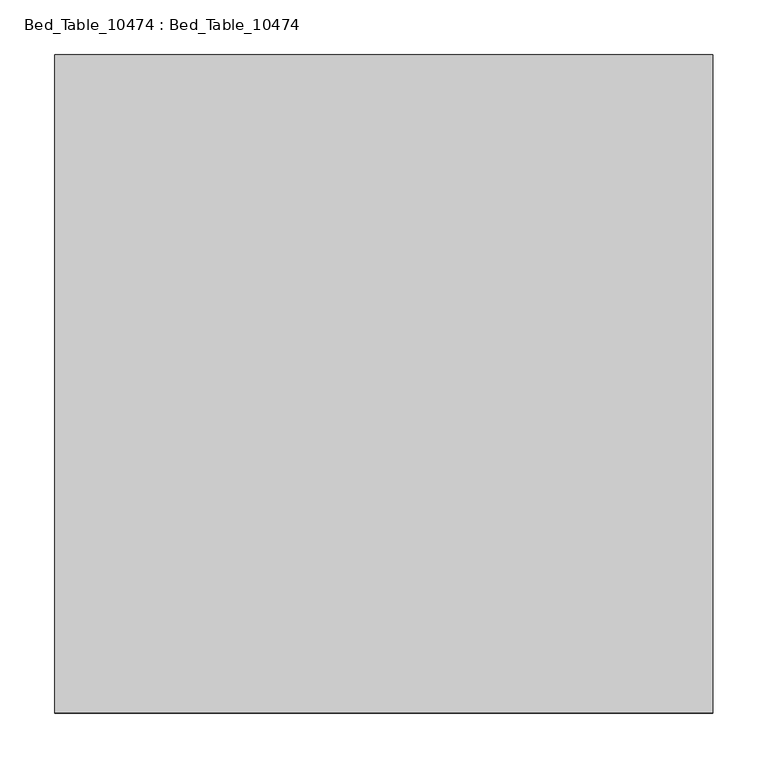
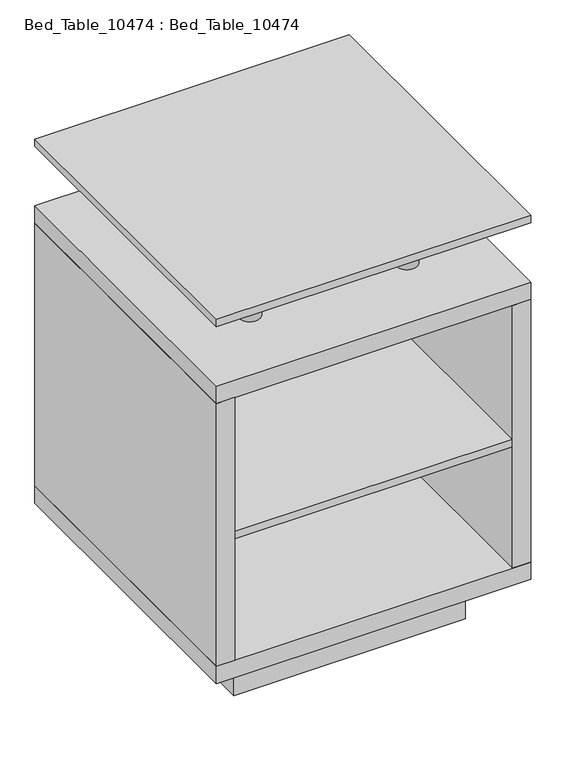
"""IFC4 building model written with IfcOpenShell, lengths in millimetres: furniture geometry, Bed_Table_10474 : Bed_Table_10474."""

from ifc_helpers import new_model, si_unit, point, frame, frame_2d, origin, origin_with_axes, place, context, project, spatial, polyline, circle_curve, trimmed, segment, composite_curve, outline, extrude, source, transform, mapped, element, save


def bed_table_10474_bed_table_10474_76a96b03(model_context):
    return source(origin(), model_context, "Body", "SweptSolid", [
        extrude(outline(polyline([(-265.0, -300.0), (-300.0, -300.0), (-300.0, 300.0), (-265.0, 300.0), (-265.0, -300.0)])), frame((0.0, 0.0, 135.0), z_axis=(0.0, 0.0, 1.0), x_axis=(1.0, 0.0, 0.0)), (0.0, 0.0, 1.0), 530.0),
        extrude(outline(polyline([(300.0, -300.0), (-300.0, -300.0), (-300.0, 300.0), (300.0, 300.0), (300.0, -300.0)])), frame((0.0, 0.0, 100.0), z_axis=(0.0, 0.0, 1.0), x_axis=(1.0, 0.0, 0.0)), (0.0, 0.0, 1.0), 35.0),
        extrude(outline(polyline([(300.0, -300.0), (-300.0, -300.0), (-300.0, 300.0), (300.0, 300.0), (300.0, -300.0)])), frame((0.0, 0.0, 665.0), z_axis=(0.0, 0.0, 1.0), x_axis=(1.0, 0.0, 0.0)), (0.0, 0.0, 1.0), 35.0),
        extrude(outline(polyline([(300.0, -300.0), (265.0, -300.0), (265.0, 300.0), (300.0, 300.0), (300.0, -300.0)])), frame((0.0, 0.0, 135.0), z_axis=(0.0, 0.0, 1.0), x_axis=(1.0, 0.0, 0.0)), (0.0, 0.0, 1.0), 530.0),
        extrude(outline(composite_curve([segment(trimmed(circle_curve(frame_2d((-150.0, -150.0)), 20.0), [point((-170.0, -150.0))], [point((-130.0, -150.0))], False, "CARTESIAN"), True, "CONTINUOUS"), segment(trimmed(circle_curve(frame_2d((-150.0, -150.0)), 20.0), [point((-130.0, -150.0))], [point((-170.0, -150.0))], False, "CARTESIAN"), True, "CONTINUOUS")], self_intersect=False)), frame((0.0, 0.0, 700.0), z_axis=(0.0, 0.0, 1.0), x_axis=(1.0, 0.0, 0.0)), (0.0, 0.0, 1.0), 120.0),
        extrude(outline(composite_curve([segment(trimmed(circle_curve(frame_2d((150.0, -150.0)), 20.0), [point((130.0, -150.0))], [point((170.0, -150.0))], False, "CARTESIAN"), True, "CONTINUOUS"), segment(trimmed(circle_curve(frame_2d((150.0, -150.0)), 20.0), [point((170.0, -150.0))], [point((130.0, -150.0))], False, "CARTESIAN"), True, "CONTINUOUS")], self_intersect=False)), frame((0.0, 0.0, 700.0), z_axis=(0.0, 0.0, 1.0), x_axis=(1.0, 0.0, 0.0)), (0.0, 0.0, 1.0), 120.0),
        extrude(outline(composite_curve([segment(trimmed(circle_curve(frame_2d((-150.0, 150.0)), 20.0), [point((-170.0, 150.0))], [point((-130.0, 150.0))], False, "CARTESIAN"), True, "CONTINUOUS"), segment(trimmed(circle_curve(frame_2d((-150.0, 150.0)), 20.0), [point((-130.0, 150.0))], [point((-170.0, 150.0))], False, "CARTESIAN"), True, "CONTINUOUS")], self_intersect=False)), frame((0.0, 0.0, 700.0), z_axis=(0.0, 0.0, 1.0), x_axis=(1.0, 0.0, 0.0)), (0.0, 0.0, 1.0), 120.0),
        extrude(outline(composite_curve([segment(trimmed(circle_curve(frame_2d((150.0, 150.0)), 20.0), [point((130.0, 150.0))], [point((170.0, 150.0))], False, "CARTESIAN"), True, "CONTINUOUS"), segment(trimmed(circle_curve(frame_2d((150.0, 150.0)), 20.0), [point((170.0, 150.0))], [point((130.0, 150.0))], False, "CARTESIAN"), True, "CONTINUOUS")], self_intersect=False)), frame((0.0, 0.0, 700.0), z_axis=(0.0, 0.0, 1.0), x_axis=(1.0, 0.0, 0.0)), (0.0, 0.0, 1.0), 120.0),
        extrude(outline(polyline([(300.0, -300.0), (-300.0, -300.0), (-300.0, 300.0), (300.0, 300.0), (300.0, -300.0)])), frame((0.0, 0.0, 820.0), z_axis=(0.0, 0.0, 1.0), x_axis=(1.0, 0.0, 0.0)), (0.0, 0.0, 1.0), 15.0),
        extrude(outline(polyline([(265.0, -300.0), (-265.0, -300.0), (-265.0, 300.0), (265.0, 300.0), (265.0, -300.0)])), frame((0.0, 0.0, 380.0), z_axis=(0.0, 0.0, 1.0), x_axis=(1.0, 0.0, 0.0)), (0.0, 0.0, 1.0), 15.0),
        extrude(outline(composite_curve([segment(trimmed(circle_curve(frame_2d((-150.0, -150.0)), 20.0), [point((-170.0, -150.0))], [point((-130.0, -150.0))], False, "CARTESIAN"), True, "CONTINUOUS"), segment(trimmed(circle_curve(frame_2d((-150.0, -150.0)), 20.0), [point((-130.0, -150.0))], [point((-170.0, -150.0))], False, "CARTESIAN"), True, "CONTINUOUS")], self_intersect=False)), origin_with_axes(), (0.0, 0.0, 1.0), 100.0),
        extrude(outline(composite_curve([segment(trimmed(circle_curve(frame_2d((150.0, -150.0)), 20.0), [point((130.0, -150.0))], [point((170.0, -150.0))], False, "CARTESIAN"), True, "CONTINUOUS"), segment(trimmed(circle_curve(frame_2d((150.0, -150.0)), 20.0), [point((170.0, -150.0))], [point((130.0, -150.0))], False, "CARTESIAN"), True, "CONTINUOUS")], self_intersect=False)), origin_with_axes(), (0.0, 0.0, 1.0), 100.0),
        extrude(outline(composite_curve([segment(trimmed(circle_curve(frame_2d((-150.0, 150.0)), 20.0), [point((-170.0, 150.0))], [point((-130.0, 150.0))], False, "CARTESIAN"), True, "CONTINUOUS"), segment(trimmed(circle_curve(frame_2d((-150.0, 150.0)), 20.0), [point((-130.0, 150.0))], [point((-170.0, 150.0))], False, "CARTESIAN"), True, "CONTINUOUS")], self_intersect=False)), origin_with_axes(), (0.0, 0.0, 1.0), 100.0),
        extrude(outline(composite_curve([segment(trimmed(circle_curve(frame_2d((150.0, 150.0)), 20.0), [point((130.0, 150.0))], [point((170.0, 150.0))], False, "CARTESIAN"), True, "CONTINUOUS"), segment(trimmed(circle_curve(frame_2d((150.0, 150.0)), 20.0), [point((170.0, 150.0))], [point((130.0, 150.0))], False, "CARTESIAN"), True, "CONTINUOUS")], self_intersect=False)), origin_with_axes(), (0.0, 0.0, 1.0), 100.0),
        extrude(outline(polyline([(-220.7106781, -220.7106781), (-220.7106781, 220.7106781), (220.7106781, 220.7106781), (220.7106781, -220.7106781), (-220.7106781, -220.7106781)]), holes=[polyline([(-210.7106781, -210.7106781), (210.7106781, -210.7106781), (210.7106781, 210.7106781), (-210.7106781, 210.7106781), (-210.7106781, -210.7106781)])]), origin_with_axes(), (0.0, 0.0, 1.0), 100.0),
    ])


if __name__ == "__main__":
    model = new_model("IFC4")
    model_context = context("Model", 3, world=origin())
    ifc_project = project(units=[si_unit("LENGTHUNIT", "METRE", prefix="MILLI")], contexts=[model_context])
    site = spatial("IfcSite", under=ifc_project)
    building = spatial("IfcBuilding", under=site)
    placement = place(None, origin())
    bed_table_10474_bed_table_10474_shape = bed_table_10474_bed_table_10474_76a96b03(model_context)
    element("IfcFurniture", 1, ObjectType="Bed_Table_10474 : Bed_Table_10474", at=placement, inside=building, context=model_context, shape_type="MappedRepresentation", body=[
        mapped(bed_table_10474_bed_table_10474_shape, transform((0.0, 0.0, 0.0), x_axis=(1.0, 0.0, 0.0), y_axis=(0.0, 1.0, 0.0), z_axis=(0.0, 0.0, 1.0))),
    ])
    save(model, "model.ifc")

# Revit data of these elements
# Type "Bed_Table_10474 : Bed_Table_10474"
#   myf = ""
#   Default Elevation = 0
# Element 1 (IfcFurniture, "Bed_Table_10474 : Bed_Table_10474")
#   Materials on its faces: "metal table", "madera", "glass table"
# Materials
#   "metal table": class "Metal", colour RGB 168 168 168, transparency 0
#   "madera": class "Wood", colour RGB 191 159 105, transparency 0
#   "glass table": class "Glass", colour RGB 229 191 0, transparency 0.95
